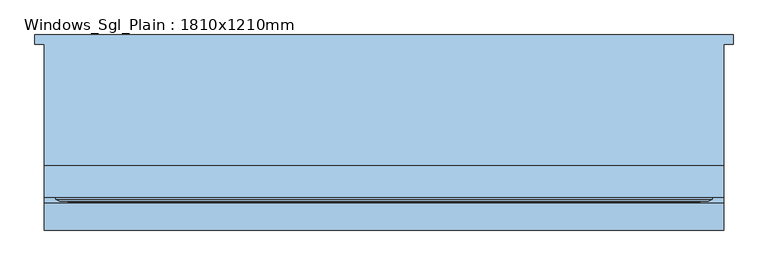
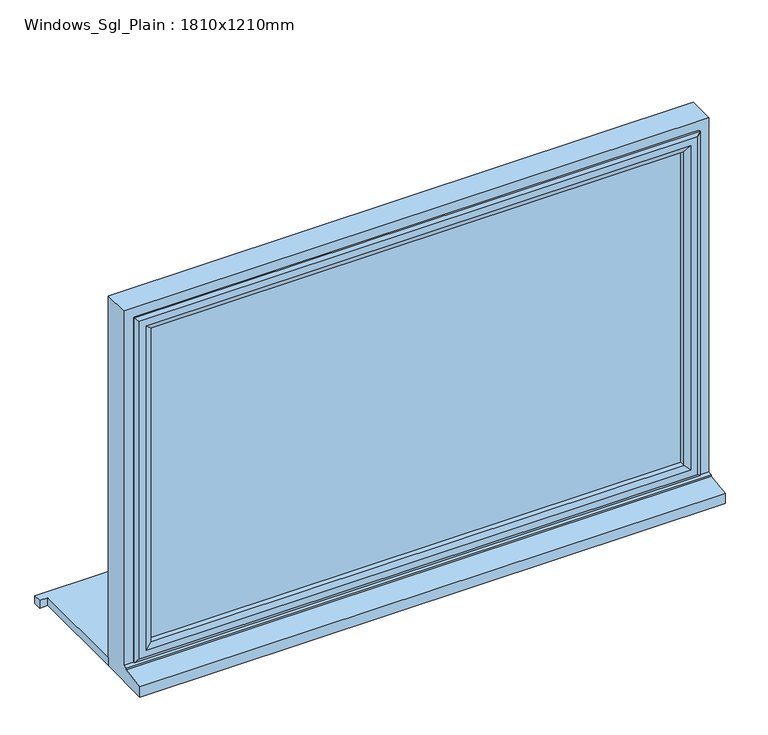
"""IFC4 building model written with IfcOpenShell, lengths in millimetres: window geometry, Windows_Sgl_Plain : 1810x1210mm."""

from ifc_helpers import new_model, si_unit, frame, origin, place, context, project, spatial, polyline, outline, extrude, faceted_brep, source, transform, mapped, element, save


def windows_sgl_plain_1810x1210mm_8b4574cd(model_context):
    return source(origin(), model_context, "Body", "SolidModel", [
        extrude(outline(polyline([(-930.0, 245.1434322), (930.0, 245.1434322), (930.0, 220.1434322), (905.0, 220.1434322), (905.0, -104.0565678), (-905.0, -104.0565678), (-905.0, 220.1434322), (-930.0, 220.1434322), (-930.0, 245.1434322)])), frame((0.0, 0.0, 900.0), z_axis=(0.0, 0.0, 1.0), x_axis=(1.0, 0.0, 0.0)), (0.0, 0.0, 1.0), 25.0),
        faceted_brep([(-905.0, -104.0565678, 900.0), (-905.0, -104.0565678, 2110.0), (905.0, -104.0565678, 2110.0), (905.0, -104.0565678, 900.0), (-845.0, -104.0565678, 2050.0), (-845.0, -104.0565678, 975.0), (845.0, -104.0565678, 975.0), (845.0, -104.0565678, 2050.0), (-905.0, -274.5565678, 900.0), (-905.0, -274.5565678, 933.8088847), (-905.0, -202.0565678, 944.7449676), (-905.0, -202.0565678, 949.68767), (-905.0, -187.0565678, 951.0), (-905.0, -187.0565678, 2110.0), (905.0, -187.0565678, 951.0), (905.0, -187.0565678, 2110.0), (-865.0, -187.0565678, 2070.0), (865.0, -187.0565678, 2070.0), (865.0, -187.0565678, 963.0), (-865.0, -187.0565678, 963.0), (-865.0, -122.0565678, 963.0), (-865.0, -122.0565678, 2070.0), (865.0, -122.0565678, 963.0), (865.0, -122.0565678, 2070.0), (-845.0, -122.0565678, 2050.0), (845.0, -122.0565678, 2050.0), (845.0, -122.0565678, 975.0), (-845.0, -122.0565678, 975.0), (905.0, -202.0565678, 949.68767), (905.0, -202.0565678, 944.7449676), (905.0, -274.5565678, 933.8088847), (905.0, -274.5565678, 900.0)], [[[0, 1, 2, 3], [4, 5, 6, 7]], [[0, 8, 9, 10, 11, 12, 13, 1]], [[12, 14, 15, 13], [16, 17, 18, 19]], [[19, 20, 21, 16]], [[21, 20, 22, 23], [24, 25, 26, 27]], [[24, 27, 5, 4]], [[1, 13, 15, 2]], [[16, 21, 23, 17]], [[7, 25, 24, 4]], [[14, 28, 29, 30, 31, 3, 2, 15]], [[17, 23, 22, 18]], [[7, 6, 26, 25]], [[31, 8, 0, 3]], [[30, 9, 8, 31]], [[29, 10, 9, 30]], [[28, 11, 10, 29]], [[14, 12, 11, 28]], [[20, 19, 18, 22]], [[5, 27, 26, 6]]]),
        extrude(outline(polyline([(835.0, -151.0565678), (835.0, -175.0565678), (-835.0, -175.0565678), (-835.0, -151.0565678), (835.0, -151.0565678)])), frame((0.0, 0.0, 993.0), z_axis=(0.0, 0.0, 1.0), x_axis=(1.0, 0.0, 0.0)), (0.0, 0.0, 1.0), 1047.0),
        faceted_brep([(-875.0, -187.0565678, 2080.0), (-875.0, -187.0565678, 953.0), (-875.0, -192.8300705, 953.0), (-875.0, -192.8300705, 2080.0), (-865.0, -122.0565678, 2070.0), (-865.0, -122.0565678, 963.0), (-865.0, -187.0565678, 963.0), (-865.0, -187.0565678, 2070.0), (-825.0, -136.5494677, 2030.0), (-825.0, -136.5494677, 1003.0), (-835.1480377, -122.0565678, 992.8519623), (-835.1480377, -122.0565678, 2040.1480377), (-825.0, -151.0565678, 2030.0), (-825.0, -151.0565678, 1003.0), (-835.0, -175.0565678, 2040.0), (-835.0, -175.0565678, 993.0), (-835.0, -151.0565678, 993.0), (-835.0, -151.0565678, 2040.0), (-825.0, -192.8300705, 2030.0), (-825.0, -192.8300705, 1003.0), (-825.0, -175.0565678, 1003.0), (-825.0, -175.0565678, 2030.0), (-842.4457548, -198.6035732, 2047.4457548), (-842.4457548, -198.6035732, 985.5542452), (-864.2153903, -198.6035732, 963.7846097), (-864.2153903, -198.6035732, 2069.2153903), (875.0, -187.0565678, 953.0), (875.0, -192.8300705, 953.0), (865.0, -122.0565678, 963.0), (865.0, -187.0565678, 963.0), (825.0, -136.5494677, 1003.0), (835.1480377, -122.0565678, 992.8519623), (825.0, -151.0565678, 1003.0), (835.0, -175.0565678, 993.0), (835.0, -151.0565678, 993.0), (825.0, -192.8300705, 1003.0), (825.0, -175.0565678, 1003.0), (842.4457548, -198.6035732, 985.5542452), (864.2153903, -198.6035732, 963.7846097), (875.0, -187.0565678, 2080.0), (875.0, -192.8300705, 2080.0), (865.0, -122.0565678, 2070.0), (865.0, -187.0565678, 2070.0), (825.0, -136.5494677, 2030.0), (835.1480377, -122.0565678, 2040.1480377), (825.0, -151.0565678, 2030.0), (835.0, -175.0565678, 2040.0), (835.0, -151.0565678, 2040.0), (825.0, -192.8300705, 2030.0), (825.0, -175.0565678, 2030.0), (842.4457548, -198.6035732, 2047.4457548), (864.2153903, -198.6035732, 2069.2153903)], [[[0, 1, 2, 3]], [[4, 5, 6, 7]], [[8, 9, 10, 11]], [[12, 13, 9, 8]], [[14, 15, 16, 17]], [[18, 19, 20, 21]], [[22, 23, 19, 18]], [[3, 2, 24, 25]], [[1, 26, 27, 2]], [[5, 28, 29, 6]], [[9, 30, 31, 10]], [[13, 32, 30, 9]], [[15, 33, 34, 16]], [[19, 35, 36, 20]], [[23, 37, 35, 19]], [[2, 27, 38, 24]], [[26, 39, 40, 27]], [[28, 41, 42, 29]], [[30, 43, 44, 31]], [[32, 45, 43, 30]], [[33, 46, 47, 34]], [[35, 48, 49, 36]], [[37, 50, 48, 35]], [[27, 40, 51, 38]], [[39, 0, 3, 40]], [[1, 0, 39, 26], [7, 6, 29, 42]], [[41, 4, 7, 42]], [[5, 4, 41, 28], [11, 10, 31, 44]], [[43, 8, 11, 44]], [[45, 12, 8, 43]], [[17, 16, 34, 47], [13, 12, 45, 32]], [[46, 14, 17, 47]], [[15, 14, 46, 33], [21, 20, 36, 49]], [[48, 18, 21, 49]], [[50, 22, 18, 48]], [[25, 24, 38, 51], [23, 22, 50, 37]], [[40, 3, 25, 51]]]),
    ])


if __name__ == "__main__":
    model = new_model("IFC4")
    model_context = context("Model", 3, world=origin())
    ifc_project = project(units=[si_unit("LENGTHUNIT", "METRE", prefix="MILLI")], contexts=[model_context])
    site = spatial("IfcSite", under=ifc_project)
    building = spatial("IfcBuilding", under=site)
    placement = place(None, origin())
    windows_sgl_plain_1810x1210mm_shape = windows_sgl_plain_1810x1210mm_8b4574cd(model_context)
    element("IfcWindow", 1, ObjectType="Windows_Sgl_Plain : 1810x1210mm", at=placement, inside=building, context=model_context, shape_type="MappedRepresentation", body=[
        mapped(windows_sgl_plain_1810x1210mm_shape, transform((0.0, 0.0, 0.0), x_axis=(1.0, 0.0, 0.0), y_axis=(0.0, 1.0, 0.0), z_axis=(0.0, 0.0, 1.0))),
    ])
    save(model, "model.ifc")

# Revit data of these elements
# Type "Windows_Sgl_Plain : 1810x1210mm"
#   Type Mark = "49"
#   Operation = "SinglePanel"
#   Construction Type Id = "SGL"
#   Manufacturer = "Revit"
#   Keynote = "L10"
#   Analytic Construction = "Large single-glazed windows"
#   Wrap Layers (Ext) from Ext = 102.5 mm
#   Wrap Layers (Int) from Ext = 177.5 mm
#   Window Board Projection = 25 mm
#   Window Board Extension = 25 mm
#   Visual Light Transmittance = 0.9
#   Solar Heat Gain Coefficient = 0.86
#   Rough Width = 1810 mm
#   Rough Height = 1210 mm
#   Height = 1210 mm
#   Width = 1810 mm
#   Heat Transfer Coefficient (U) = 5.5617 W/(m²·K)
#   Glazing Thickness = 24 mm
#   FrameOffset - External = 50 mm
#   Frame Depth = 65 mm
#   Default Head Height = 2110 mm
#   Cill Depth = 87.5 mm
#   Cavity Closer Width = 50 mm
#   Cavity Closer Offset from Ext = 102.5 mm
#   Cavity Closer Depth = 85 mm
#   Define Thermal Properties by = 1
#   Vis - Cavity Closers = yes
#   Define Thermal Properties by = 1
#   Material Trim = Window Frame
#   Material Glass = Glass
#   Material Frame = Window Frame
#   Wall Closure = (empty or 0)
# Element 1 (IfcWindow, "Windows_Sgl_Plain : 1810x1210mm")
#   Materials on its faces: "Window Frame", "Glass"
# Materials
#   "Window Frame": colour RGB 249 249 249, transparency 0, Keynote = "L10", Cost = 0
#   "Glass": class "Glass", colour RGB 0 128 192, transparency 0.9, Description = "Soda Lime Glass", Cost = 0
